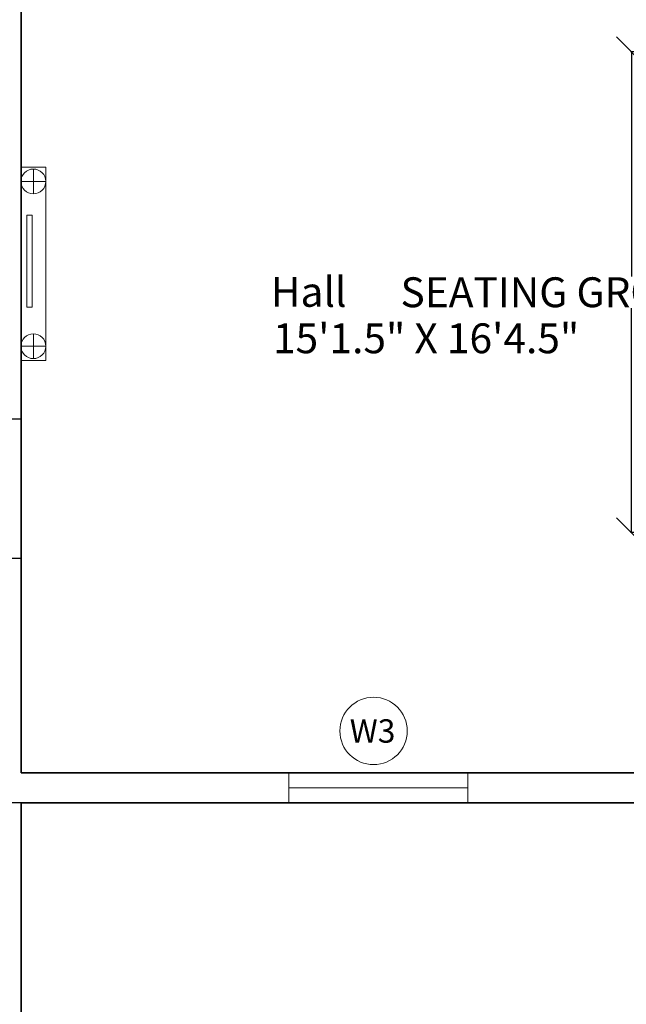
# Model space of a CAD drawing. Units: inches. Extents: x -1198 to -69, y -512 to 437.
# Tile 42 of 50: x -566 to -444, y -85 to 113. Entities that reach past the tile are written whole.
import ezdxf

# ---------------------------------------------------------------- set-up
doc = ezdxf.new("R2010")
doc.units = ezdxf.units.IN
doc.header["$MEASUREMENT"] = 0
for name, color, linetype, lineweight in [('A-ANNO-DIMS', 2, 'Continuous', 18), ('A-ANNO-SYMB', 7, 'Continuous', 18), ('A-AREA-IDEN', 7, 'Continuous', 18), ('A-EQPM', 60, 'Continuous', 18), ('A-WALL', 7, 'Continuous', 35), ('Doors', 140, 'Continuous', 25), ('windows', 160, 'Continuous', 18)]:
    doc.layers.add(name, color=color, linetype=linetype, lineweight=lineweight)
doc.styles.get("Standard").update_dxf_attribs({"font": 'arial.ttf'})
doc.dimstyles.get("Standard").update_dxf_attribs({"dimtxt": 6, "dimasz": 6, "dimexe": 0.18, "dimexo": 0.0625, "dimgap": 0.09, "dimtad": 0, "dimtih": 1, "dimtoh": 1, "dimdec": 0, "dimzin": 0, "dimdsep": 46, "dimlunit": 4, "dimtxsty": 'Standard', "dimblk": 'OBLIQUE', "dimcen": 0.09, "dimadec": 0, "dimazin": 0, "dimtfac": 1, "dimtdec": 0, "dimtofl": 0, "dimtmove": 0, "dimatfit": 3, "dimfxl": 1, "dimtolj": 1, "dimtzin": 0, "dimarcsym": 0})

# ---------------------------------------------------------------- blocks, each defined once
blk = doc.blocks.new('*U4')
for p, q in [((0, 0), (0, -6)), ((28, 0), (28, -6))]:
    blk.add_line(p, q)
blk.add_lwpolyline([(0, 0), (0, 28), (1.75, 28), (1.75, 0)], close=True)
blk.add_arc((0, 0), 28, 0, 90)
blk = doc.blocks.new('WIN-W3-36')
at = {"ltscale": 10}
for p, q in [((0, 6), (0, 0)), ((36, 6), (36, 0)), ((0, 3), (36, 3))]:
    blk.add_line(p, q, dxfattribs=at)
blk = doc.blocks.new('TV-CONSOLE')
at = {"ltscale": 10}
for p, q in [((2.49, 33.45), (2.49, 38.43)), ((4.97, 35.94), (0, 35.94)), ((2.49, 5.34), (2.49, 0.37)), ((4.97, 2.85), (0, 2.85))]:
    blk.add_line(p, q, dxfattribs=at)
for points in [[(4.97, 38.79), (0, 38.79), (0, 0), (4.97, 0)], [(2.27, 29.19), (1.16, 29.19), (1.16, 10.69), (2.27, 10.69)]]:
    blk.add_lwpolyline(points, close=True, dxfattribs=at)
for centre in [(2.49, 35.94), (2.49, 2.85)]:
    blk.add_circle(centre, 2.49, dxfattribs=at)
blk = doc.blocks.new('TAG-W3')
at = {"ltscale": 10}
blk.add_circle((0, 0), 6.77, dxfattribs=at)
blk.add_text('W3', height=4.7, dxfattribs=at).set_placement((-4.79, -2.36))
blk = doc.blocks.new('_Oblique')
at = {"color": 0, "linetype": 'ByBlock', "lineweight": -2}
blk.add_line((-0.5, -0.5), (0.5, 0.5), dxfattribs=at)
blk = doc.blocks.new('*D52')
at = {"layer": 'A-ANNO-DIMS', "color": 0, "lineweight": -2, "ltscale": 10, "transparency": 16777216}
for p, q in [((-428.65, 106.55), (-443.25, 106.55)), ((-443.07, 106.55), (-443.07, 61.46)), ((-443.07, 9.98), (-443.07, 55.07)), ((-428.65, 9.98), (-443.25, 9.98))]:
    blk.add_line(p, q, dxfattribs=at)
at = {"layer": 'DEFPOINTS', "color": 0, "ltscale": 10, "transparency": 16777216}
for p in [(-428.58, 106.55), (-443.07, 9.98), (-428.58, 9.98)]:
    blk.add_point(p, dxfattribs=at)
at = {"layer": 'A-ANNO-DIMS', "color": 0, "lineweight": -2, "ltscale": 10, "transparency": 16777216, "xscale": 6, "yscale": 6, "zscale": 6}
for p, rotation in [((-443.07, 106.55), 90), ((-443.07, 9.98), 270)]:
    blk.add_blockref('_Oblique', p, dxfattribs=dict(at, rotation=rotation))
at = {"layer": 'A-ANNO-DIMS', "color": 0, "ltscale": 10, "transparency": 16777216, "insert": (-443.07, 58.27), "char_height": 6, "attachment_point": 5}
blk.add_mtext('\\A1;SEATING GROUP 97 TYP.', dxfattribs=at)
blk = doc.blocks.new('*D75')
at = {"layer": 'A-ANNO-DIMS', "color": 0, "lineweight": -2, "ltscale": 10, "transparency": 16777216}
for p, q in [((-376.81, -44.27), (-1188.2, -44.27)), ((-1188.02, -44.27), (-1188.02, -133.37)), ((-1188.02, -228.77), (-1188.02, -139.68)), ((-370.81, -228.77), (-1188.2, -228.77))]:
    blk.add_line(p, q, dxfattribs=at)
at = {"layer": 'DEFPOINTS', "color": 0, "ltscale": 10, "transparency": 16777216}
for p in [(-1188.02, -44.27), (-376.75, -44.27), (-370.75, -228.77)]:
    blk.add_point(p, dxfattribs=at)
at = {"layer": 'A-ANNO-DIMS', "color": 0, "lineweight": -2, "ltscale": 10, "transparency": 16777216, "xscale": 6, "yscale": 6, "zscale": 6}
for p, rotation in [((-1188.02, -44.27), 90), ((-1188.02, -228.77), 270)]:
    blk.add_blockref('_Oblique', p, dxfattribs=dict(at, rotation=rotation))
at = {"layer": 'A-ANNO-DIMS', "color": 0, "ltscale": 10, "transparency": 16777216, "insert": (-1188.02, -136.52), "char_height": 6, "attachment_point": 5}
blk.add_mtext('\\A1;184.5', dxfattribs=at)

msp = doc.modelspace()

# ---------------------------------------------------------------- linework, layer by layer
at = {"layer": 'A-WALL', "ltscale": 10}
for p, q in [((-565.7509, 161.2277), (-565.7509, 35.2277)), ((-565.7509, 35.2277), (-565.7509, -38.2723)), ((-422.1319, -38.2723), (-565.7509, -38.2723)), ((-565.7509, -44.2723), (-565.7509, -125.2723)), ((-376.7509, -44.2723), (-565.7509, -44.2723))]:
    msp.add_line(p, q, dxfattribs=at)

# ---------------------------------------------------------------- block references
at = {"layer": 'A-ANNO-SYMB'}
msp.add_blockref('TAG-W3', (-494.8941, -29.8595), dxfattribs=at)
at = {"layer": 'A-EQPM'}
msp.add_blockref('TV-CONSOLE', (-565.751, 44.584), dxfattribs=at)
at = {"layer": 'Doors', "xscale": -1, "rotation": 90}
msp.add_blockref('*U4', (-571.7509, 32.874), dxfattribs=at)
at = {"layer": 'windows'}
msp.add_blockref('WIN-W3-36', (-511.941, -44.272), dxfattribs=at)

# ---------------------------------------------------------------- texts
at = {"layer": 'A-AREA-IDEN', "ltscale": 10, "char_height": 6, "attachment_point": 1}
for s, width, insert in [('Hall', 57.976527, (-515.5351, 61.3442)), ('15\'1.5" X 16\'4.5"', 62.175425, (-515.1157, 52.0171))]:
    msp.add_mtext_dynamic_manual_height_columns(s, width=width, gutter_width=30, heights=[0], dxfattribs=dict(at, insert=insert))

# ---------------------------------------------------------------- dimensions: what is measured, and where the dimension line sits
at = {"layer": 'A-ANNO-DIMS', "ltscale": 10}
dim = msp.add_linear_dim(base=(-443.0692, 9.981), p1=(-428.5837, 106.551), p2=(-428.5837, 9.981), angle=270, text='SEATING GROUP <> TYP.', dimstyle='Standard', override={"dimdec": 0, "dimlfac": 1, "dimrnd": 0, "dimzin": 0, "dimdsep": 46, "dimlunit": 2}, dxfattribs=at)
dim.commit()
dim.dimension.update_dxf_attribs({"geometry": '*D52', "text_midpoint": (-443.0692, 58.266)})
dim = msp.add_linear_dim(base=(-1188.0248, -44.2723), p1=(-370.7509, -228.7723), p2=(-376.7509, -44.2723), angle=90, dimstyle='Standard', override={"dimdec": 1, "dimlfac": 1, "dimrnd": 0, "dimzin": 0, "dimdsep": 46, "dimlunit": 2}, dxfattribs=at)
dim.commit()
dim.dimension.update_dxf_attribs({"geometry": '*D75', "text_midpoint": (-1188.0248, -136.5223)})

doc.saveas('drawing.dxf')
